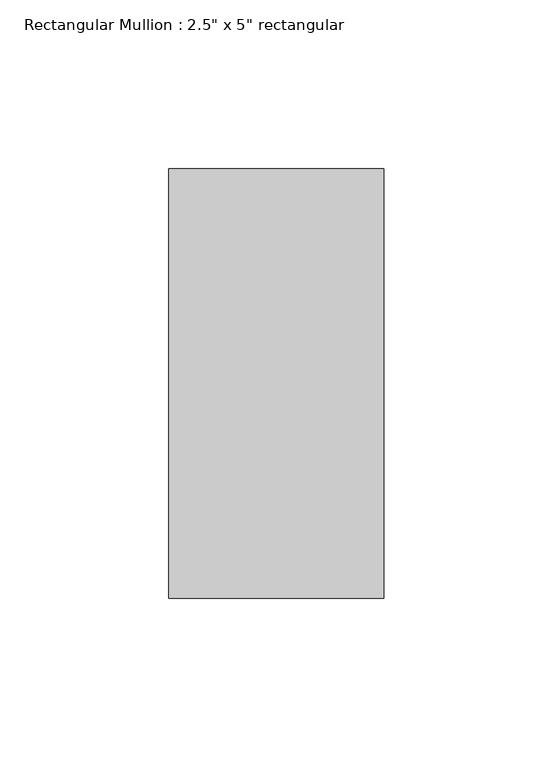
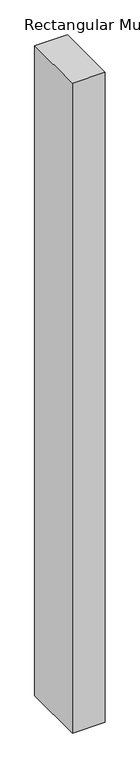
"""IFC4 building model written with IfcOpenShell, lengths in millimetres: member geometry."""

from ifc_helpers import new_model, si_unit, frame, origin, place, context, project, spatial, polyline, outline, extrude, source, transform, mapped, element, save


def member_37150780(model_context):
    return source(origin(), model_context, "Body", "SweptSolid", [
        extrude(outline(polyline([(31.75, 63.5), (31.75, -63.5), (-31.75, -63.5), (-31.75, 63.5), (31.75, 63.5)])), frame((0.0, 0.0, -1333.4999998), z_axis=(0.0, 0.0, 1.0), x_axis=(1.0, 0.0, 0.0)), (0.0, 0.0, 1.0), 1333.4999998),
    ])


if __name__ == "__main__":
    model = new_model("IFC4")
    model_context = context("Model", 3, world=origin())
    ifc_project = project(units=[si_unit("LENGTHUNIT", "METRE", prefix="MILLI")], contexts=[model_context])
    site = spatial("IfcSite", under=ifc_project)
    building = spatial("IfcBuilding", under=site)
    placement = place(None, origin())
    member_shape = member_37150780(model_context)
    element("IfcMember", 1, ObjectType="Rectangular Mullion : 2.5\" x 5\" rectangular", at=placement, inside=building, context=model_context, shape_type="MappedRepresentation", body=[
        mapped(member_shape, transform((0.0, 0.0, 0.0), x_axis=(1.0, 0.0, 0.0), y_axis=(0.0, 1.0, 0.0), z_axis=(0.0, 0.0, 1.0))),
    ])
    save(model, "model.ifc")

# Revit data of these elements
# Type "Rectangular Mullion : 2.5\" x 5\" rectangular"
#   built-in parameter 1007304 = 0.416667 (stored number, unit not read)
#   built-in parameter 1007301 = 0.104167 (stored number, unit not read)
#   built-in parameter 1007300 = 0.104167 (stored number, unit not read)
# Element 1 (IfcMember, "Rectangular Mullion : 2.5\" x 5\" rectangular")
#   Materials on its faces: "Aluminum"
# Materials
#   "Aluminum": class "Metal", colour RGB 247 247 247, transparency 0, Description = "Aluminum 6061", Cost = 0
